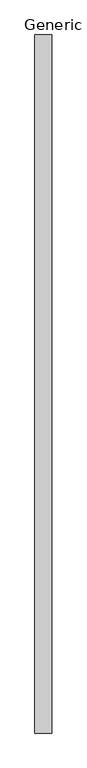
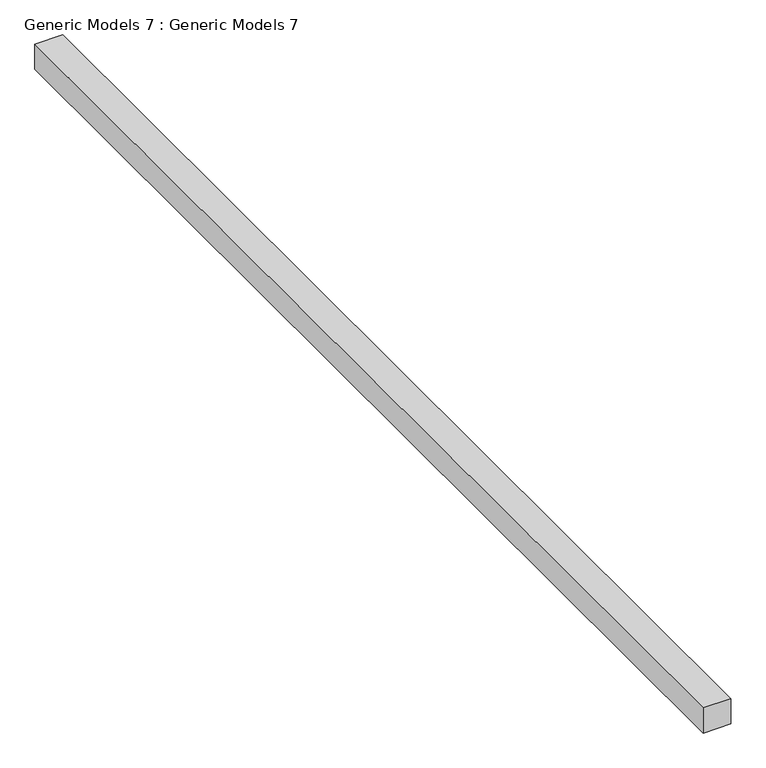
"""IFC4 building model written with IfcOpenShell, lengths in millimetres: proxy geometry, Generic Models 7 : Generic Models 7."""

from ifc_helpers import new_model, si_unit, frame, origin, place, context, project, spatial, polyline, outline, extrude, source, transform, mapped, element, save


def generic_models_7_generic_models_7_7f11944a(model_context):
    return source(origin(), model_context, "Body", "SweptSolid", [
        extrude(outline(polyline([(-15581.438074, -5922.3713044), (-15581.438074, 6778.7941506), (-15276.638074, 6778.7941506), (-15276.638074, -5922.3713044), (-15581.438074, -5922.3713044)])), frame((0.0, 0.0, 36271.2), z_axis=(0.0, 0.0, 1.0), x_axis=(1.0, 0.0, 0.0)), (0.0, 0.0, 1.0), 292.0195447),
    ])


if __name__ == "__main__":
    model = new_model("IFC4")
    model_context = context("Model", 3, world=origin())
    ifc_project = project(units=[si_unit("LENGTHUNIT", "METRE", prefix="MILLI")], contexts=[model_context])
    site = spatial("IfcSite", under=ifc_project)
    building = spatial("IfcBuilding", under=site)
    placement = place(None, origin())
    generic_models_7_generic_models_7_shape = generic_models_7_generic_models_7_7f11944a(model_context)
    element("IfcBuildingElementProxy", 1, Name="Generic Models 7 : Generic Models 7", ObjectType="Generic Models 7 : Generic Models 7", at=placement, inside=building, context=model_context, shape_type="MappedRepresentation", body=[
        mapped(generic_models_7_generic_models_7_shape, transform((0.0, 0.0, 0.0), x_axis=(1.0, 0.0, 0.0), y_axis=(0.0, 1.0, 0.0), z_axis=(0.0, 0.0, 1.0))),
    ])
    save(model, "model.ifc")
